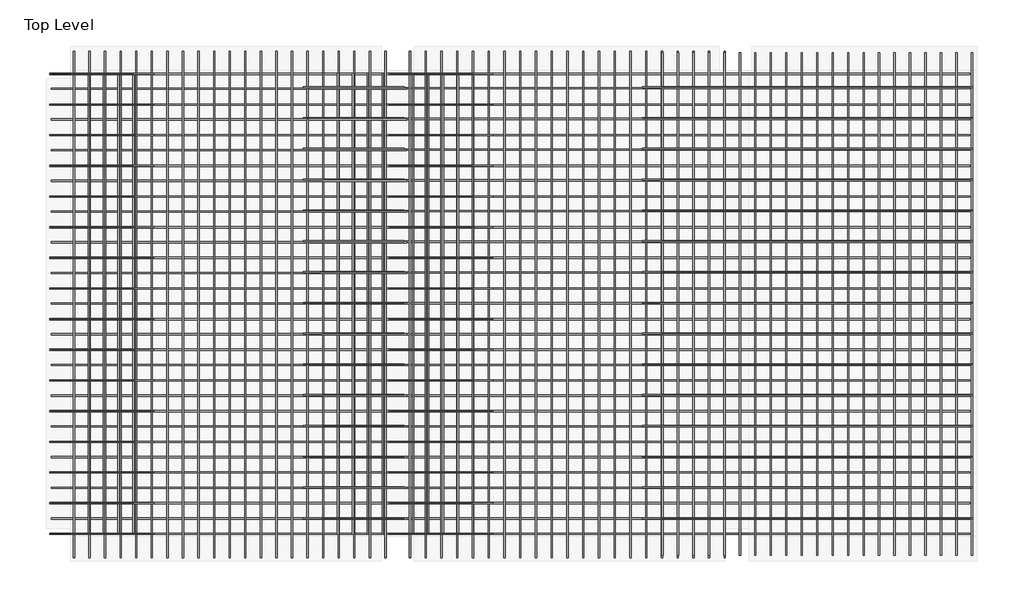
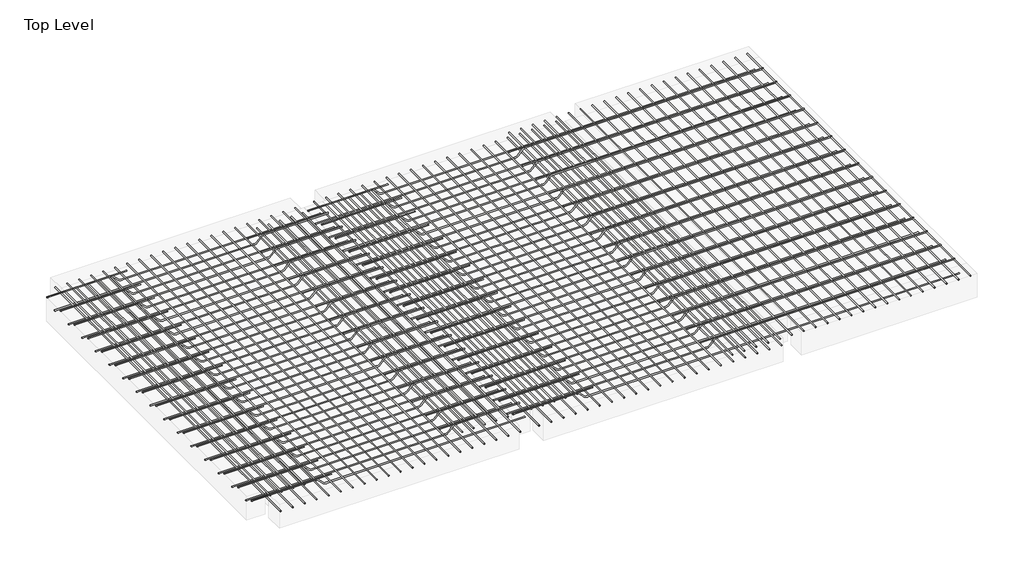
# One storey, part 2 of 2: 14 reinforcing bars.
"""IFC4 building model written with IfcOpenShell, lengths in millimetres."""

from ifc_helpers import new_model, si_unit, point, frame, origin, place, context, project, spatial, polyline, circle_curve, trimmed, segment, composite_curve, source, transform, mapped, element, save
from ifc_brep_helpers import swept_disk

model = new_model("IFC4")

# Units and contexts
model_context = context("Model", 3, world=origin())
ifc_project = project(units=[si_unit("LENGTHUNIT", "METRE", prefix="MILLI")], contexts=[model_context])

# Site, building, storey
site = spatial("IfcSite", under=ifc_project)
building = spatial("IfcBuilding", under=site)
storey = spatial("IfcBuildingStorey", under=building, Name="Top Level", Elevation=12801.6)

# Reinforcing bars
placement = place(None, origin())
reinforcing_bar_shape = source(origin(), model_context, "Body", "SolidModel", [
    swept_disk(composite_curve([segment(polyline([(-9347.5125695, 4803.6334631, 12770.6), (-8565.5792829, 4803.6334631, 12770.6)]), True, "CONTINUOUS"), segment(trimmed(circle_curve(frame((-8565.5792829, 4803.6334631, 12724.6), z_axis=(0.0, 1.0, 0.0), x_axis=(0.0, 0.0, 46.0)), 46.0), [point((-8565.5792829, 4803.6334631, 12770.6))], [point((-8533.052371, 4803.6334631, 12757.1269119))], True, "CARTESIAN"), True, "CONTINUOUS"), segment(polyline([(-8533.052371, 4803.6334631, 12757.1269119), (-8469.5985471, 4803.6334631, 12693.6730881)]), True, "CONTINUOUS"), segment(trimmed(circle_curve(frame((-8437.0716352, 4803.6334631, 12726.2), z_axis=(0.0, -1.0000000000000002, 0.0), x_axis=(-32.526911900000414, 0.0, -32.526911900000414)), 46.0), [point((-8469.5985471, 4803.6334631, 12693.6730881))], [point((-8437.0716352, 4803.6334631, 12680.2))], True, "CARTESIAN"), True, "CONTINUOUS"), segment(polyline([(-8437.0716352, 4803.6334631, 12680.2), (-5982.0597449, 4803.6334631, 12680.2)]), True, "CONTINUOUS")], self_intersect=False), 6.0),
])
element("IfcReinforcingBar", 1, at=placement, inside=storey, context=model_context, shape_type="MappedRepresentation", body=[
    mapped(reinforcing_bar_shape, transform((0.0, 0.0, 0.0), x_axis=(1.0, 0.0, 0.0), y_axis=(0.0, 1.0, 0.0), z_axis=(0.0, 0.0, 1.0))),
    mapped(reinforcing_bar_shape, transform((0.0, -290.5066667, 0.0), x_axis=(1.0, 0.0, 0.0), y_axis=(0.0, 1.0, 0.0), z_axis=(0.0, 0.0, 1.0))),
    mapped(reinforcing_bar_shape, transform((0.0, -581.0133333, 0.0), x_axis=(1.0, 0.0, 0.0), y_axis=(0.0, 1.0, 0.0), z_axis=(0.0, 0.0, 1.0))),
    mapped(reinforcing_bar_shape, transform((0.0, -871.52, 0.0), x_axis=(1.0, 0.0, 0.0), y_axis=(0.0, 1.0, 0.0), z_axis=(0.0, 0.0, 1.0))),
    mapped(reinforcing_bar_shape, transform((0.0, -1162.0266667, 0.0), x_axis=(1.0, 0.0, 0.0), y_axis=(0.0, 1.0, 0.0), z_axis=(0.0, 0.0, 1.0))),
    mapped(reinforcing_bar_shape, transform((0.0, -1452.5333333, 0.0), x_axis=(1.0, 0.0, 0.0), y_axis=(0.0, 1.0, 0.0), z_axis=(0.0, 0.0, 1.0))),
    mapped(reinforcing_bar_shape, transform((0.0, -1743.04, 0.0), x_axis=(1.0, 0.0, 0.0), y_axis=(0.0, 1.0, 0.0), z_axis=(0.0, 0.0, 1.0))),
    mapped(reinforcing_bar_shape, transform((0.0, -2033.5466667, 0.0), x_axis=(1.0, 0.0, 0.0), y_axis=(0.0, 1.0, 0.0), z_axis=(0.0, 0.0, 1.0))),
    mapped(reinforcing_bar_shape, transform((0.0, -2324.0533333, 0.0), x_axis=(1.0, 0.0, 0.0), y_axis=(0.0, 1.0, 0.0), z_axis=(0.0, 0.0, 1.0))),
    mapped(reinforcing_bar_shape, transform((0.0, -2614.56, 0.0), x_axis=(1.0, 0.0, 0.0), y_axis=(0.0, 1.0, 0.0), z_axis=(0.0, 0.0, 1.0))),
    mapped(reinforcing_bar_shape, transform((0.0, -2905.0666667, 0.0), x_axis=(1.0, 0.0, 0.0), y_axis=(0.0, 1.0, 0.0), z_axis=(0.0, 0.0, 1.0))),
    mapped(reinforcing_bar_shape, transform((0.0, -3195.5733333, 0.0), x_axis=(1.0, 0.0, 0.0), y_axis=(0.0, 1.0, 0.0), z_axis=(0.0, 0.0, 1.0))),
    mapped(reinforcing_bar_shape, transform((0.0, -3486.08, 0.0), x_axis=(1.0, 0.0, 0.0), y_axis=(0.0, 1.0, 0.0), z_axis=(0.0, 0.0, 1.0))),
    mapped(reinforcing_bar_shape, transform((0.0, -3776.5866667, 0.0), x_axis=(1.0, 0.0, 0.0), y_axis=(0.0, 1.0, 0.0), z_axis=(0.0, 0.0, 1.0))),
    mapped(reinforcing_bar_shape, transform((0.0, -4067.0933333, 0.0), x_axis=(1.0, 0.0, 0.0), y_axis=(0.0, 1.0, 0.0), z_axis=(0.0, 0.0, 1.0))),
    mapped(reinforcing_bar_shape, transform((0.0, -4357.6, 0.0), x_axis=(1.0, 0.0, 0.0), y_axis=(0.0, 1.0, 0.0), z_axis=(0.0, 0.0, 1.0))),
])
reinforcing_bar_2_shape = source(origin(), model_context, "Body", "SolidModel", [
    swept_disk(composite_curve([segment(polyline([(-5968.6109354, 590.4513536, 12770.6), (-6750.544222, 590.4513536, 12770.6)]), True, "CONTINUOUS"), segment(trimmed(circle_curve(frame((-6750.544222, 590.4513536, 12724.6), z_axis=(0.0, -1.0, 0.0), x_axis=(0.0, 0.0, 46.0)), 46.0), [point((-6750.544222, 590.4513536, 12770.6))], [point((-6783.0711339, 590.4513536, 12757.1269119))], True, "CARTESIAN"), True, "CONTINUOUS"), segment(polyline([(-6783.0711339, 590.4513536, 12757.1269119), (-6846.5249578, 590.4513536, 12693.6730881)]), True, "CONTINUOUS"), segment(trimmed(circle_curve(frame((-6879.0518697, 590.4513536, 12726.2), z_axis=(0.0, 1.0000000000000002, 0.0), x_axis=(32.526911899999504, 0.0, -32.526911900000414)), 46.0), [point((-6846.5249578, 590.4513536, 12693.6730881))], [point((-6879.0518697, 590.4513536, 12680.2))], True, "CARTESIAN"), True, "CONTINUOUS"), segment(polyline([(-6879.0518697, 590.4513536, 12680.2), (-9334.06376, 590.4513536, 12680.2)]), True, "CONTINUOUS")], self_intersect=False), 6.0),
])
element("IfcReinforcingBar", 2, at=placement, inside=storey, context=model_context, shape_type="MappedRepresentation", body=[
    mapped(reinforcing_bar_2_shape, transform((0.0, 0.0, 0.0), x_axis=(1.0, 0.0, 0.0), y_axis=(0.0, 1.0, 0.0), z_axis=(0.0, 0.0, 1.0))),
    mapped(reinforcing_bar_2_shape, transform((0.0, 290.9296088, 0.0), x_axis=(1.0, 0.0, 0.0), y_axis=(0.0, 1.0, 0.0), z_axis=(0.0, 0.0, 1.0))),
    mapped(reinforcing_bar_2_shape, transform((0.0, 581.8592177, 0.0), x_axis=(1.0, 0.0, 0.0), y_axis=(0.0, 1.0, 0.0), z_axis=(0.0, 0.0, 1.0))),
    mapped(reinforcing_bar_2_shape, transform((0.0, 872.7888265, 0.0), x_axis=(1.0, 0.0, 0.0), y_axis=(0.0, 1.0, 0.0), z_axis=(0.0, 0.0, 1.0))),
    mapped(reinforcing_bar_2_shape, transform((0.0, 1163.7184353, 0.0), x_axis=(1.0, 0.0, 0.0), y_axis=(0.0, 1.0, 0.0), z_axis=(0.0, 0.0, 1.0))),
    mapped(reinforcing_bar_2_shape, transform((0.0, 1454.6480442, 0.0), x_axis=(1.0, 0.0, 0.0), y_axis=(0.0, 1.0, 0.0), z_axis=(0.0, 0.0, 1.0))),
    mapped(reinforcing_bar_2_shape, transform((0.0, 1745.577653, 0.0), x_axis=(1.0, 0.0, 0.0), y_axis=(0.0, 1.0, 0.0), z_axis=(0.0, 0.0, 1.0))),
    mapped(reinforcing_bar_2_shape, transform((0.0, 2036.5072618, 0.0), x_axis=(1.0, 0.0, 0.0), y_axis=(0.0, 1.0, 0.0), z_axis=(0.0, 0.0, 1.0))),
    mapped(reinforcing_bar_2_shape, transform((0.0, 2327.4368707, 0.0), x_axis=(1.0, 0.0, 0.0), y_axis=(0.0, 1.0, 0.0), z_axis=(0.0, 0.0, 1.0))),
    mapped(reinforcing_bar_2_shape, transform((0.0, 2618.3664795, 0.0), x_axis=(1.0, 0.0, 0.0), y_axis=(0.0, 1.0, 0.0), z_axis=(0.0, 0.0, 1.0))),
    mapped(reinforcing_bar_2_shape, transform((0.0, 2909.2960883, 0.0), x_axis=(1.0, 0.0, 0.0), y_axis=(0.0, 1.0, 0.0), z_axis=(0.0, 0.0, 1.0))),
    mapped(reinforcing_bar_2_shape, transform((0.0, 3200.2256972, 0.0), x_axis=(1.0, 0.0, 0.0), y_axis=(0.0, 1.0, 0.0), z_axis=(0.0, 0.0, 1.0))),
    mapped(reinforcing_bar_2_shape, transform((0.0, 3491.155306, 0.0), x_axis=(1.0, 0.0, 0.0), y_axis=(0.0, 1.0, 0.0), z_axis=(0.0, 0.0, 1.0))),
    mapped(reinforcing_bar_2_shape, transform((0.0, 3782.0849148, 0.0), x_axis=(1.0, 0.0, 0.0), y_axis=(0.0, 1.0, 0.0), z_axis=(0.0, 0.0, 1.0))),
    mapped(reinforcing_bar_2_shape, transform((0.0, 4073.0145236, 0.0), x_axis=(1.0, 0.0, 0.0), y_axis=(0.0, 1.0, 0.0), z_axis=(0.0, 0.0, 1.0))),
])
reinforcing_bar_3_shape = source(origin(), model_context, "Body", "SolidModel", [
    swept_disk(composite_curve([segment(polyline([(-8556.5984173, 4809.6334631, 12760.3006995), (-8556.5984173, 440.0334631, 12760.3006995)]), True, "CONTINUOUS")], self_intersect=False), 6.0),
])
element("IfcReinforcingBar", 3, at=placement, inside=storey, context=model_context, shape_type="MappedRepresentation", body=[
    mapped(reinforcing_bar_3_shape, transform((0.0, 0.0, 0.0), x_axis=(1.0, 0.0, 0.0), y_axis=(0.0, 1.0, 0.0), z_axis=(0.0, 0.0, 1.0))),
    mapped(reinforcing_bar_3_shape, transform((-140.6783338, 0.0, 0.0), x_axis=(1.0, 0.0, 0.0), y_axis=(0.0, 1.0, 0.0), z_axis=(0.0, 0.0, 1.0))),
    mapped(reinforcing_bar_3_shape, transform((-281.3566676, 0.0, 0.0), x_axis=(1.0, 0.0, 0.0), y_axis=(0.0, 1.0, 0.0), z_axis=(0.0, 0.0, 1.0))),
    mapped(reinforcing_bar_3_shape, transform((-422.0350014, 0.0, 0.0), x_axis=(1.0, 0.0, 0.0), y_axis=(0.0, 1.0, 0.0), z_axis=(0.0, 0.0, 1.0))),
    mapped(reinforcing_bar_3_shape, transform((-562.7133352, 0.0, 0.0), x_axis=(1.0, 0.0, 0.0), y_axis=(0.0, 1.0, 0.0), z_axis=(0.0, 0.0, 1.0))),
])
reinforcing_bar_4_shape = source(origin(), model_context, "Body", "SolidModel", [
    swept_disk(composite_curve([segment(polyline([(-6759.5250876, 4809.6334631, 12760.3006995), (-6759.5250876, 440.0334631, 12760.3006995)]), True, "CONTINUOUS")], self_intersect=False), 6.0),
])
element("IfcReinforcingBar", 4, at=placement, inside=storey, context=model_context, shape_type="MappedRepresentation", body=[
    mapped(reinforcing_bar_4_shape, transform((0.0, 0.0, 0.0), x_axis=(1.0, 0.0, 0.0), y_axis=(0.0, 1.0, 0.0), z_axis=(0.0, 0.0, 1.0))),
    mapped(reinforcing_bar_4_shape, transform((140.6783338, 0.0, 0.0), x_axis=(1.0, 0.0, 0.0), y_axis=(0.0, 1.0, 0.0), z_axis=(0.0, 0.0, 1.0))),
    mapped(reinforcing_bar_4_shape, transform((281.3566676, 0.0, 0.0), x_axis=(1.0, 0.0, 0.0), y_axis=(0.0, 1.0, 0.0), z_axis=(0.0, 0.0, 1.0))),
    mapped(reinforcing_bar_4_shape, transform((422.0350014, 0.0, 0.0), x_axis=(1.0, 0.0, 0.0), y_axis=(0.0, 1.0, 0.0), z_axis=(0.0, 0.0, 1.0))),
    mapped(reinforcing_bar_4_shape, transform((562.7133352, 0.0, 0.0), x_axis=(1.0, 0.0, 0.0), y_axis=(0.0, 1.0, 0.0), z_axis=(0.0, 0.0, 1.0))),
])
reinforcing_bar_5_shape = source(origin(), model_context, "Body", "SolidModel", [
    swept_disk(composite_curve([segment(polyline([(-9338.4522926, 4805.6334631, 12772.6), (-8365.7369752, 4805.6334631, 12772.6)]), True, "CONTINUOUS")], self_intersect=False), 4.0),
])
element("IfcReinforcingBar", 5, at=placement, inside=storey, context=model_context, shape_type="MappedRepresentation", body=[
    mapped(reinforcing_bar_5_shape, transform((0.0, 0.0, 0.0), x_axis=(1.0, 0.0, 0.0), y_axis=(0.0, 1.0, 0.0), z_axis=(0.0, 0.0, 1.0))),
    mapped(reinforcing_bar_5_shape, transform((0.0, -290.7733333, 0.0), x_axis=(1.0, 0.0, 0.0), y_axis=(0.0, 1.0, 0.0), z_axis=(0.0, 0.0, 1.0))),
    mapped(reinforcing_bar_5_shape, transform((0.0, -581.5466667, 0.0), x_axis=(1.0, 0.0, 0.0), y_axis=(0.0, 1.0, 0.0), z_axis=(0.0, 0.0, 1.0))),
    mapped(reinforcing_bar_5_shape, transform((0.0, -872.32, 0.0), x_axis=(1.0, 0.0, 0.0), y_axis=(0.0, 1.0, 0.0), z_axis=(0.0, 0.0, 1.0))),
    mapped(reinforcing_bar_5_shape, transform((0.0, -1163.0933333, 0.0), x_axis=(1.0, 0.0, 0.0), y_axis=(0.0, 1.0, 0.0), z_axis=(0.0, 0.0, 1.0))),
    mapped(reinforcing_bar_5_shape, transform((0.0, -1453.8666667, 0.0), x_axis=(1.0, 0.0, 0.0), y_axis=(0.0, 1.0, 0.0), z_axis=(0.0, 0.0, 1.0))),
    mapped(reinforcing_bar_5_shape, transform((0.0, -1744.64, 0.0), x_axis=(1.0, 0.0, 0.0), y_axis=(0.0, 1.0, 0.0), z_axis=(0.0, 0.0, 1.0))),
    mapped(reinforcing_bar_5_shape, transform((0.0, -2035.4133333, 0.0), x_axis=(1.0, 0.0, 0.0), y_axis=(0.0, 1.0, 0.0), z_axis=(0.0, 0.0, 1.0))),
    mapped(reinforcing_bar_5_shape, transform((0.0, -2326.1866667, 0.0), x_axis=(1.0, 0.0, 0.0), y_axis=(0.0, 1.0, 0.0), z_axis=(0.0, 0.0, 1.0))),
    mapped(reinforcing_bar_5_shape, transform((0.0, -2616.96, 0.0), x_axis=(1.0, 0.0, 0.0), y_axis=(0.0, 1.0, 0.0), z_axis=(0.0, 0.0, 1.0))),
    mapped(reinforcing_bar_5_shape, transform((0.0, -2907.7333333, 0.0), x_axis=(1.0, 0.0, 0.0), y_axis=(0.0, 1.0, 0.0), z_axis=(0.0, 0.0, 1.0))),
    mapped(reinforcing_bar_5_shape, transform((0.0, -3198.5066667, 0.0), x_axis=(1.0, 0.0, 0.0), y_axis=(0.0, 1.0, 0.0), z_axis=(0.0, 0.0, 1.0))),
    mapped(reinforcing_bar_5_shape, transform((0.0, -3489.28, 0.0), x_axis=(1.0, 0.0, 0.0), y_axis=(0.0, 1.0, 0.0), z_axis=(0.0, 0.0, 1.0))),
    mapped(reinforcing_bar_5_shape, transform((0.0, -3780.0533333, 0.0), x_axis=(1.0, 0.0, 0.0), y_axis=(0.0, 1.0, 0.0), z_axis=(0.0, 0.0, 1.0))),
    mapped(reinforcing_bar_5_shape, transform((0.0, -4070.8266667, 0.0), x_axis=(1.0, 0.0, 0.0), y_axis=(0.0, 1.0, 0.0), z_axis=(0.0, 0.0, 1.0))),
    mapped(reinforcing_bar_5_shape, transform((0.0, -4361.6, 0.0), x_axis=(1.0, 0.0, 0.0), y_axis=(0.0, 1.0, 0.0), z_axis=(0.0, 0.0, 1.0))),
])
reinforcing_bar_6_shape = source(origin(), model_context, "Body", "SolidModel", [
    swept_disk(composite_curve([segment(polyline([(-5991.3123639, 4678.4115375, 12772.6), (-6950.3865297, 4678.4115375, 12772.6)]), True, "CONTINUOUS")], self_intersect=False), 4.0),
])
element("IfcReinforcingBar", 6, at=placement, inside=storey, context=model_context, shape_type="MappedRepresentation", body=[
    mapped(reinforcing_bar_6_shape, transform((0.0, 0.0, 0.0), x_axis=(1.0, 0.0, 0.0), y_axis=(0.0, 1.0, 0.0), z_axis=(0.0, 0.0, 1.0))),
    mapped(reinforcing_bar_6_shape, transform((0.0, -291.8025106, 0.0), x_axis=(1.0, 0.0, 0.0), y_axis=(0.0, 1.0, 0.0), z_axis=(0.0, 0.0, 1.0))),
    mapped(reinforcing_bar_6_shape, transform((0.0, -583.6050212, 0.0), x_axis=(1.0, 0.0, 0.0), y_axis=(0.0, 1.0, 0.0), z_axis=(0.0, 0.0, 1.0))),
    mapped(reinforcing_bar_6_shape, transform((0.0, -875.4075319, 0.0), x_axis=(1.0, 0.0, 0.0), y_axis=(0.0, 1.0, 0.0), z_axis=(0.0, 0.0, 1.0))),
    mapped(reinforcing_bar_6_shape, transform((0.0, -1167.2100425, 0.0), x_axis=(1.0, 0.0, 0.0), y_axis=(0.0, 1.0, 0.0), z_axis=(0.0, 0.0, 1.0))),
    mapped(reinforcing_bar_6_shape, transform((0.0, -1459.0125531, 0.0), x_axis=(1.0, 0.0, 0.0), y_axis=(0.0, 1.0, 0.0), z_axis=(0.0, 0.0, 1.0))),
    mapped(reinforcing_bar_6_shape, transform((0.0, -1750.8150637, 0.0), x_axis=(1.0, 0.0, 0.0), y_axis=(0.0, 1.0, 0.0), z_axis=(0.0, 0.0, 1.0))),
    mapped(reinforcing_bar_6_shape, transform((0.0, -2042.6175743, 0.0), x_axis=(1.0, 0.0, 0.0), y_axis=(0.0, 1.0, 0.0), z_axis=(0.0, 0.0, 1.0))),
    mapped(reinforcing_bar_6_shape, transform((0.0, -2334.420085, 0.0), x_axis=(1.0, 0.0, 0.0), y_axis=(0.0, 1.0, 0.0), z_axis=(0.0, 0.0, 1.0))),
    mapped(reinforcing_bar_6_shape, transform((0.0, -2626.2225956, 0.0), x_axis=(1.0, 0.0, 0.0), y_axis=(0.0, 1.0, 0.0), z_axis=(0.0, 0.0, 1.0))),
    mapped(reinforcing_bar_6_shape, transform((0.0, -2918.0251062, 0.0), x_axis=(1.0, 0.0, 0.0), y_axis=(0.0, 1.0, 0.0), z_axis=(0.0, 0.0, 1.0))),
    mapped(reinforcing_bar_6_shape, transform((0.0, -3209.8276168, 0.0), x_axis=(1.0, 0.0, 0.0), y_axis=(0.0, 1.0, 0.0), z_axis=(0.0, 0.0, 1.0))),
    mapped(reinforcing_bar_6_shape, transform((0.0, -3501.6301274, 0.0), x_axis=(1.0, 0.0, 0.0), y_axis=(0.0, 1.0, 0.0), z_axis=(0.0, 0.0, 1.0))),
    mapped(reinforcing_bar_6_shape, transform((0.0, -3793.4326381, 0.0), x_axis=(1.0, 0.0, 0.0), y_axis=(0.0, 1.0, 0.0), z_axis=(0.0, 0.0, 1.0))),
    mapped(reinforcing_bar_6_shape, transform((0.0, -4085.2351487, 0.0), x_axis=(1.0, 0.0, 0.0), y_axis=(0.0, 1.0, 0.0), z_axis=(0.0, 0.0, 1.0))),
])
reinforcing_bar_7_shape = source(origin(), model_context, "Body", "SolidModel", [
    swept_disk(composite_curve([segment(polyline([(-6169.8117524, 218.9117605, 12688.7387401), (-6169.8117524, 5019.9992064, 12688.7387401)]), True, "CONTINUOUS")], self_intersect=False), 6.0),
])
element("IfcReinforcingBar", 7, at=placement, inside=storey, context=model_context, shape_type="MappedRepresentation", body=[
    mapped(reinforcing_bar_7_shape, transform((0.0, 0.0, 0.0), x_axis=(1.0, 0.0, 0.0), y_axis=(0.0, 1.0, 0.0), z_axis=(0.0, 0.0, 1.0))),
    mapped(reinforcing_bar_7_shape, transform((-147.475, 0.0, 0.0), x_axis=(1.0, 0.0, 0.0), y_axis=(0.0, 1.0, 0.0), z_axis=(0.0, 0.0, 1.0))),
    mapped(reinforcing_bar_7_shape, transform((-294.95, 0.0, 0.0), x_axis=(1.0, 0.0, 0.0), y_axis=(0.0, 1.0, 0.0), z_axis=(0.0, 0.0, 1.0))),
    mapped(reinforcing_bar_7_shape, transform((-442.425, 0.0, 0.0), x_axis=(1.0, 0.0, 0.0), y_axis=(0.0, 1.0, 0.0), z_axis=(0.0, 0.0, 1.0))),
    mapped(reinforcing_bar_7_shape, transform((-589.9, 0.0, 0.0), x_axis=(1.0, 0.0, 0.0), y_axis=(0.0, 1.0, 0.0), z_axis=(0.0, 0.0, 1.0))),
    mapped(reinforcing_bar_7_shape, transform((-737.375, 0.0, 0.0), x_axis=(1.0, 0.0, 0.0), y_axis=(0.0, 1.0, 0.0), z_axis=(0.0, 0.0, 1.0))),
    mapped(reinforcing_bar_7_shape, transform((-884.85, 0.0, 0.0), x_axis=(1.0, 0.0, 0.0), y_axis=(0.0, 1.0, 0.0), z_axis=(0.0, 0.0, 1.0))),
    mapped(reinforcing_bar_7_shape, transform((-1032.325, 0.0, 0.0), x_axis=(1.0, 0.0, 0.0), y_axis=(0.0, 1.0, 0.0), z_axis=(0.0, 0.0, 1.0))),
    mapped(reinforcing_bar_7_shape, transform((-1179.8, 0.0, 0.0), x_axis=(1.0, 0.0, 0.0), y_axis=(0.0, 1.0, 0.0), z_axis=(0.0, 0.0, 1.0))),
    mapped(reinforcing_bar_7_shape, transform((-1327.275, 0.0, 0.0), x_axis=(1.0, 0.0, 0.0), y_axis=(0.0, 1.0, 0.0), z_axis=(0.0, 0.0, 1.0))),
    mapped(reinforcing_bar_7_shape, transform((-1474.75, 0.0, 0.0), x_axis=(1.0, 0.0, 0.0), y_axis=(0.0, 1.0, 0.0), z_axis=(0.0, 0.0, 1.0))),
    mapped(reinforcing_bar_7_shape, transform((-1622.225, 0.0, 0.0), x_axis=(1.0, 0.0, 0.0), y_axis=(0.0, 1.0, 0.0), z_axis=(0.0, 0.0, 1.0))),
    mapped(reinforcing_bar_7_shape, transform((-1769.7, 0.0, 0.0), x_axis=(1.0, 0.0, 0.0), y_axis=(0.0, 1.0, 0.0), z_axis=(0.0, 0.0, 1.0))),
    mapped(reinforcing_bar_7_shape, transform((-1917.175, 0.0, 0.0), x_axis=(1.0, 0.0, 0.0), y_axis=(0.0, 1.0, 0.0), z_axis=(0.0, 0.0, 1.0))),
    mapped(reinforcing_bar_7_shape, transform((-2064.65, 0.0, 0.0), x_axis=(1.0, 0.0, 0.0), y_axis=(0.0, 1.0, 0.0), z_axis=(0.0, 0.0, 1.0))),
    mapped(reinforcing_bar_7_shape, transform((-2212.125, 0.0, 0.0), x_axis=(1.0, 0.0, 0.0), y_axis=(0.0, 1.0, 0.0), z_axis=(0.0, 0.0, 1.0))),
    mapped(reinforcing_bar_7_shape, transform((-2359.6, 0.0, 0.0), x_axis=(1.0, 0.0, 0.0), y_axis=(0.0, 1.0, 0.0), z_axis=(0.0, 0.0, 1.0))),
    mapped(reinforcing_bar_7_shape, transform((-2507.075, 0.0, 0.0), x_axis=(1.0, 0.0, 0.0), y_axis=(0.0, 1.0, 0.0), z_axis=(0.0, 0.0, 1.0))),
    mapped(reinforcing_bar_7_shape, transform((-2654.55, 0.0, 0.0), x_axis=(1.0, 0.0, 0.0), y_axis=(0.0, 1.0, 0.0), z_axis=(0.0, 0.0, 1.0))),
    mapped(reinforcing_bar_7_shape, transform((-2802.025, 0.0, 0.0), x_axis=(1.0, 0.0, 0.0), y_axis=(0.0, 1.0, 0.0), z_axis=(0.0, 0.0, 1.0))),
    mapped(reinforcing_bar_7_shape, transform((-2949.5, 0.0, 0.0), x_axis=(1.0, 0.0, 0.0), y_axis=(0.0, 1.0, 0.0), z_axis=(0.0, 0.0, 1.0))),
])
reinforcing_bar_8_shape = source(origin(), model_context, "Body", "SolidModel", [
    swept_disk(composite_curve([segment(polyline([(-6134.4125695, 4803.6334631, 12770.6), (-5352.4792829, 4803.6334631, 12770.6)]), True, "CONTINUOUS"), segment(trimmed(circle_curve(frame((-5352.4792829, 4803.6334631, 12724.6), z_axis=(0.0, 1.0, 0.0), x_axis=(0.0, 0.0, 46.0)), 46.0), [point((-5352.4792829, 4803.6334631, 12770.6))], [point((-5319.952371, 4803.6334631, 12757.1269119))], True, "CARTESIAN"), True, "CONTINUOUS"), segment(polyline([(-5319.952371, 4803.6334631, 12757.1269119), (-5256.4985471, 4803.6334631, 12693.6730881)]), True, "CONTINUOUS"), segment(trimmed(circle_curve(frame((-5223.9716352, 4803.6334631, 12726.2), z_axis=(0.0, -1.0, 0.0), x_axis=(-32.526911900000414, 0.0, -32.526911900000414)), 46.0), [point((-5256.4985471, 4803.6334631, 12693.6730881))], [point((-5223.9716352, 4803.6334631, 12680.2))], True, "CARTESIAN"), True, "CONTINUOUS"), segment(polyline([(-5223.9716352, 4803.6334631, 12680.2), (-639.5382507, 4803.6334631, 12680.2)]), True, "CONTINUOUS")], self_intersect=False), 6.0),
])
element("IfcReinforcingBar", 8, at=placement, inside=storey, context=model_context, shape_type="MappedRepresentation", body=[
    mapped(reinforcing_bar_8_shape, transform((0.0, 0.0, 0.0), x_axis=(1.0, 0.0, 0.0), y_axis=(0.0, 1.0, 0.0), z_axis=(0.0, 0.0, 1.0))),
    mapped(reinforcing_bar_8_shape, transform((0.0, -290.5066667, 0.0), x_axis=(1.0, 0.0, 0.0), y_axis=(0.0, 1.0, 0.0), z_axis=(0.0, 0.0, 1.0))),
    mapped(reinforcing_bar_8_shape, transform((0.0, -581.0133333, 0.0), x_axis=(1.0, 0.0, 0.0), y_axis=(0.0, 1.0, 0.0), z_axis=(0.0, 0.0, 1.0))),
    mapped(reinforcing_bar_8_shape, transform((0.0, -871.52, 0.0), x_axis=(1.0, 0.0, 0.0), y_axis=(0.0, 1.0, 0.0), z_axis=(0.0, 0.0, 1.0))),
    mapped(reinforcing_bar_8_shape, transform((0.0, -1162.0266667, 0.0), x_axis=(1.0, 0.0, 0.0), y_axis=(0.0, 1.0, 0.0), z_axis=(0.0, 0.0, 1.0))),
    mapped(reinforcing_bar_8_shape, transform((0.0, -1452.5333333, 0.0), x_axis=(1.0, 0.0, 0.0), y_axis=(0.0, 1.0, 0.0), z_axis=(0.0, 0.0, 1.0))),
    mapped(reinforcing_bar_8_shape, transform((0.0, -1743.04, 0.0), x_axis=(1.0, 0.0, 0.0), y_axis=(0.0, 1.0, 0.0), z_axis=(0.0, 0.0, 1.0))),
    mapped(reinforcing_bar_8_shape, transform((0.0, -2033.5466667, 0.0), x_axis=(1.0, 0.0, 0.0), y_axis=(0.0, 1.0, 0.0), z_axis=(0.0, 0.0, 1.0))),
    mapped(reinforcing_bar_8_shape, transform((0.0, -2324.0533333, 0.0), x_axis=(1.0, 0.0, 0.0), y_axis=(0.0, 1.0, 0.0), z_axis=(0.0, 0.0, 1.0))),
    mapped(reinforcing_bar_8_shape, transform((0.0, -2614.56, 0.0), x_axis=(1.0, 0.0, 0.0), y_axis=(0.0, 1.0, 0.0), z_axis=(0.0, 0.0, 1.0))),
    mapped(reinforcing_bar_8_shape, transform((0.0, -2905.0666667, 0.0), x_axis=(1.0, 0.0, 0.0), y_axis=(0.0, 1.0, 0.0), z_axis=(0.0, 0.0, 1.0))),
    mapped(reinforcing_bar_8_shape, transform((0.0, -3195.5733333, 0.0), x_axis=(1.0, 0.0, 0.0), y_axis=(0.0, 1.0, 0.0), z_axis=(0.0, 0.0, 1.0))),
    mapped(reinforcing_bar_8_shape, transform((0.0, -3486.08, 0.0), x_axis=(1.0, 0.0, 0.0), y_axis=(0.0, 1.0, 0.0), z_axis=(0.0, 0.0, 1.0))),
    mapped(reinforcing_bar_8_shape, transform((0.0, -3776.5866667, 0.0), x_axis=(1.0, 0.0, 0.0), y_axis=(0.0, 1.0, 0.0), z_axis=(0.0, 0.0, 1.0))),
    mapped(reinforcing_bar_8_shape, transform((0.0, -4067.0933333, 0.0), x_axis=(1.0, 0.0, 0.0), y_axis=(0.0, 1.0, 0.0), z_axis=(0.0, 0.0, 1.0))),
    mapped(reinforcing_bar_8_shape, transform((0.0, -4357.6, 0.0), x_axis=(1.0, 0.0, 0.0), y_axis=(0.0, 1.0, 0.0), z_axis=(0.0, 0.0, 1.0))),
])
reinforcing_bar_9_shape = source(origin(), model_context, "Body", "SolidModel", [
    swept_disk(composite_curve([segment(polyline([(-634.9311577, 590.4513536, 12770.6), (-3537.444222, 590.4513536, 12770.6)]), True, "CONTINUOUS"), segment(trimmed(circle_curve(frame((-3537.444222, 590.4513536, 12724.6), z_axis=(0.0, -1.0, 0.0), x_axis=(0.0, 0.0, 46.0)), 46.0), [point((-3537.444222, 590.4513536, 12770.6))], [point((-3569.9711339, 590.4513536, 12757.1269119))], True, "CARTESIAN"), True, "CONTINUOUS"), segment(polyline([(-3569.9711339, 590.4513536, 12757.1269119), (-3633.4249578, 590.4513536, 12693.6730881)]), True, "CONTINUOUS"), segment(trimmed(circle_curve(frame((-3665.9518697, 590.4513536, 12726.2), z_axis=(0.0, 1.0, 0.0), x_axis=(32.52691189999996, 0.0, -32.526911900000414)), 46.0), [point((-3633.4249578, 590.4513536, 12693.6730881))], [point((-3665.9518697, 590.4513536, 12680.2))], True, "CARTESIAN"), True, "CONTINUOUS"), segment(polyline([(-3665.9518697, 590.4513536, 12680.2), (-6120.96376, 590.4513536, 12680.2)]), True, "CONTINUOUS")], self_intersect=False), 6.0),
])
element("IfcReinforcingBar", 9, at=placement, inside=storey, context=model_context, shape_type="MappedRepresentation", body=[
    mapped(reinforcing_bar_9_shape, transform((0.0, 0.0, 0.0), x_axis=(1.0, 0.0, 0.0), y_axis=(0.0, 1.0, 0.0), z_axis=(0.0, 0.0, 1.0))),
    mapped(reinforcing_bar_9_shape, transform((0.0, 291.2629007, 0.0), x_axis=(1.0, 0.0, 0.0), y_axis=(0.0, 1.0, 0.0), z_axis=(0.0, 0.0, 1.0))),
    mapped(reinforcing_bar_9_shape, transform((0.0, 582.5258014, 0.0), x_axis=(1.0, 0.0, 0.0), y_axis=(0.0, 1.0, 0.0), z_axis=(0.0, 0.0, 1.0))),
    mapped(reinforcing_bar_9_shape, transform((0.0, 873.7887021, 0.0), x_axis=(1.0, 0.0, 0.0), y_axis=(0.0, 1.0, 0.0), z_axis=(0.0, 0.0, 1.0))),
    mapped(reinforcing_bar_9_shape, transform((0.0, 1165.0516028, 0.0), x_axis=(1.0, 0.0, 0.0), y_axis=(0.0, 1.0, 0.0), z_axis=(0.0, 0.0, 1.0))),
    mapped(reinforcing_bar_9_shape, transform((0.0, 1456.3145035, 0.0), x_axis=(1.0, 0.0, 0.0), y_axis=(0.0, 1.0, 0.0), z_axis=(0.0, 0.0, 1.0))),
    mapped(reinforcing_bar_9_shape, transform((0.0, 1747.5774042, 0.0), x_axis=(1.0, 0.0, 0.0), y_axis=(0.0, 1.0, 0.0), z_axis=(0.0, 0.0, 1.0))),
    mapped(reinforcing_bar_9_shape, transform((0.0, 2038.8403049, 0.0), x_axis=(1.0, 0.0, 0.0), y_axis=(0.0, 1.0, 0.0), z_axis=(0.0, 0.0, 1.0))),
    mapped(reinforcing_bar_9_shape, transform((0.0, 2330.1032056, 0.0), x_axis=(1.0, 0.0, 0.0), y_axis=(0.0, 1.0, 0.0), z_axis=(0.0, 0.0, 1.0))),
    mapped(reinforcing_bar_9_shape, transform((0.0, 2621.3661063, 0.0), x_axis=(1.0, 0.0, 0.0), y_axis=(0.0, 1.0, 0.0), z_axis=(0.0, 0.0, 1.0))),
    mapped(reinforcing_bar_9_shape, transform((0.0, 2912.629007, 0.0), x_axis=(1.0, 0.0, 0.0), y_axis=(0.0, 1.0, 0.0), z_axis=(0.0, 0.0, 1.0))),
    mapped(reinforcing_bar_9_shape, transform((0.0, 3203.8919077, 0.0), x_axis=(1.0, 0.0, 0.0), y_axis=(0.0, 1.0, 0.0), z_axis=(0.0, 0.0, 1.0))),
    mapped(reinforcing_bar_9_shape, transform((0.0, 3495.1548084, 0.0), x_axis=(1.0, 0.0, 0.0), y_axis=(0.0, 1.0, 0.0), z_axis=(0.0, 0.0, 1.0))),
    mapped(reinforcing_bar_9_shape, transform((0.0, 3786.4177091, 0.0), x_axis=(1.0, 0.0, 0.0), y_axis=(0.0, 1.0, 0.0), z_axis=(0.0, 0.0, 1.0))),
    mapped(reinforcing_bar_9_shape, transform((0.0, 4077.6806098, 0.0), x_axis=(1.0, 0.0, 0.0), y_axis=(0.0, 1.0, 0.0), z_axis=(0.0, 0.0, 1.0))),
])
reinforcing_bar_10_shape = source(origin(), model_context, "Body", "SolidModel", [
    swept_disk(composite_curve([segment(polyline([(-3546.4250876, 5003.4291982, 12760.3006995), (-3546.4250876, 243.4585871, 12760.3006995)]), True, "CONTINUOUS")], self_intersect=False), 6.0),
])
element("IfcReinforcingBar", 10, at=placement, inside=storey, context=model_context, shape_type="MappedRepresentation", body=[
    mapped(reinforcing_bar_10_shape, transform((0.0, 0.0, 0.0), x_axis=(1.0, 0.0, 0.0), y_axis=(0.0, 1.0, 0.0), z_axis=(0.0, 0.0, 1.0))),
    mapped(reinforcing_bar_10_shape, transform((146.4369665, 0.0, 0.0), x_axis=(1.0, 0.0, 0.0), y_axis=(0.0, 1.0, 0.0), z_axis=(0.0, 0.0, 1.0))),
    mapped(reinforcing_bar_10_shape, transform((292.8739331, 0.0, 0.0), x_axis=(1.0, 0.0, 0.0), y_axis=(0.0, 1.0, 0.0), z_axis=(0.0, 0.0, 1.0))),
    mapped(reinforcing_bar_10_shape, transform((439.3108996, 0.0, 0.0), x_axis=(1.0, 0.0, 0.0), y_axis=(0.0, 1.0, 0.0), z_axis=(0.0, 0.0, 1.0))),
    mapped(reinforcing_bar_10_shape, transform((585.7478661, 0.0, 0.0), x_axis=(1.0, 0.0, 0.0), y_axis=(0.0, 1.0, 0.0), z_axis=(0.0, 0.0, 1.0))),
    mapped(reinforcing_bar_10_shape, transform((732.1848326, 0.0, 0.0), x_axis=(1.0, 0.0, 0.0), y_axis=(0.0, 1.0, 0.0), z_axis=(0.0, 0.0, 1.0))),
    mapped(reinforcing_bar_10_shape, transform((878.6217992, 0.0, 0.0), x_axis=(1.0, 0.0, 0.0), y_axis=(0.0, 1.0, 0.0), z_axis=(0.0, 0.0, 1.0))),
    mapped(reinforcing_bar_10_shape, transform((1025.0587657, 0.0, 0.0), x_axis=(1.0, 0.0, 0.0), y_axis=(0.0, 1.0, 0.0), z_axis=(0.0, 0.0, 1.0))),
    mapped(reinforcing_bar_10_shape, transform((1171.4957322, 0.0, 0.0), x_axis=(1.0, 0.0, 0.0), y_axis=(0.0, 1.0, 0.0), z_axis=(0.0, 0.0, 1.0))),
    mapped(reinforcing_bar_10_shape, transform((1317.9326988, 0.0, 0.0), x_axis=(1.0, 0.0, 0.0), y_axis=(0.0, 1.0, 0.0), z_axis=(0.0, 0.0, 1.0))),
    mapped(reinforcing_bar_10_shape, transform((1464.3696653, 0.0, 0.0), x_axis=(1.0, 0.0, 0.0), y_axis=(0.0, 1.0, 0.0), z_axis=(0.0, 0.0, 1.0))),
    mapped(reinforcing_bar_10_shape, transform((1610.8066318, 0.0, 0.0), x_axis=(1.0, 0.0, 0.0), y_axis=(0.0, 1.0, 0.0), z_axis=(0.0, 0.0, 1.0))),
    mapped(reinforcing_bar_10_shape, transform((1757.2435983, 0.0, 0.0), x_axis=(1.0, 0.0, 0.0), y_axis=(0.0, 1.0, 0.0), z_axis=(0.0, 0.0, 1.0))),
    mapped(reinforcing_bar_10_shape, transform((1903.6805649, 0.0, 0.0), x_axis=(1.0, 0.0, 0.0), y_axis=(0.0, 1.0, 0.0), z_axis=(0.0, 0.0, 1.0))),
    mapped(reinforcing_bar_10_shape, transform((2050.1175314, 0.0, 0.0), x_axis=(1.0, 0.0, 0.0), y_axis=(0.0, 1.0, 0.0), z_axis=(0.0, 0.0, 1.0))),
    mapped(reinforcing_bar_10_shape, transform((2196.5544979, 0.0, 0.0), x_axis=(1.0, 0.0, 0.0), y_axis=(0.0, 1.0, 0.0), z_axis=(0.0, 0.0, 1.0))),
    mapped(reinforcing_bar_10_shape, transform((2342.9914645, 0.0, 0.0), x_axis=(1.0, 0.0, 0.0), y_axis=(0.0, 1.0, 0.0), z_axis=(0.0, 0.0, 1.0))),
    mapped(reinforcing_bar_10_shape, transform((2489.428431, 0.0, 0.0), x_axis=(1.0, 0.0, 0.0), y_axis=(0.0, 1.0, 0.0), z_axis=(0.0, 0.0, 1.0))),
    mapped(reinforcing_bar_10_shape, transform((2635.8653975, 0.0, 0.0), x_axis=(1.0, 0.0, 0.0), y_axis=(0.0, 1.0, 0.0), z_axis=(0.0, 0.0, 1.0))),
    mapped(reinforcing_bar_10_shape, transform((2782.302364, 0.0, 0.0), x_axis=(1.0, 0.0, 0.0), y_axis=(0.0, 1.0, 0.0), z_axis=(0.0, 0.0, 1.0))),
    mapped(reinforcing_bar_10_shape, transform((2928.7393306, 0.0, 0.0), x_axis=(1.0, 0.0, 0.0), y_axis=(0.0, 1.0, 0.0), z_axis=(0.0, 0.0, 1.0))),
])
reinforcing_bar_11_shape = source(origin(), model_context, "Body", "SolidModel", [
    swept_disk(composite_curve([segment(polyline([(-6125.3522926, 4805.6334631, 12772.6), (-5152.6369752, 4805.6334631, 12772.6)]), True, "CONTINUOUS")], self_intersect=False), 4.0),
])
element("IfcReinforcingBar", 11, at=placement, inside=storey, context=model_context, shape_type="MappedRepresentation", body=[
    mapped(reinforcing_bar_11_shape, transform((0.0, 0.0, 0.0), x_axis=(1.0, 0.0, 0.0), y_axis=(0.0, 1.0, 0.0), z_axis=(0.0, 0.0, 1.0))),
    mapped(reinforcing_bar_11_shape, transform((0.0, -290.7733333, 0.0), x_axis=(1.0, 0.0, 0.0), y_axis=(0.0, 1.0, 0.0), z_axis=(0.0, 0.0, 1.0))),
    mapped(reinforcing_bar_11_shape, transform((0.0, -581.5466667, 0.0), x_axis=(1.0, 0.0, 0.0), y_axis=(0.0, 1.0, 0.0), z_axis=(0.0, 0.0, 1.0))),
    mapped(reinforcing_bar_11_shape, transform((0.0, -872.32, 0.0), x_axis=(1.0, 0.0, 0.0), y_axis=(0.0, 1.0, 0.0), z_axis=(0.0, 0.0, 1.0))),
    mapped(reinforcing_bar_11_shape, transform((0.0, -1163.0933333, 0.0), x_axis=(1.0, 0.0, 0.0), y_axis=(0.0, 1.0, 0.0), z_axis=(0.0, 0.0, 1.0))),
    mapped(reinforcing_bar_11_shape, transform((0.0, -1453.8666667, 0.0), x_axis=(1.0, 0.0, 0.0), y_axis=(0.0, 1.0, 0.0), z_axis=(0.0, 0.0, 1.0))),
    mapped(reinforcing_bar_11_shape, transform((0.0, -1744.64, 0.0), x_axis=(1.0, 0.0, 0.0), y_axis=(0.0, 1.0, 0.0), z_axis=(0.0, 0.0, 1.0))),
    mapped(reinforcing_bar_11_shape, transform((0.0, -2035.4133333, 0.0), x_axis=(1.0, 0.0, 0.0), y_axis=(0.0, 1.0, 0.0), z_axis=(0.0, 0.0, 1.0))),
    mapped(reinforcing_bar_11_shape, transform((0.0, -2326.1866667, 0.0), x_axis=(1.0, 0.0, 0.0), y_axis=(0.0, 1.0, 0.0), z_axis=(0.0, 0.0, 1.0))),
    mapped(reinforcing_bar_11_shape, transform((0.0, -2616.96, 0.0), x_axis=(1.0, 0.0, 0.0), y_axis=(0.0, 1.0, 0.0), z_axis=(0.0, 0.0, 1.0))),
    mapped(reinforcing_bar_11_shape, transform((0.0, -2907.7333333, 0.0), x_axis=(1.0, 0.0, 0.0), y_axis=(0.0, 1.0, 0.0), z_axis=(0.0, 0.0, 1.0))),
    mapped(reinforcing_bar_11_shape, transform((0.0, -3198.5066667, 0.0), x_axis=(1.0, 0.0, 0.0), y_axis=(0.0, 1.0, 0.0), z_axis=(0.0, 0.0, 1.0))),
    mapped(reinforcing_bar_11_shape, transform((0.0, -3489.28, 0.0), x_axis=(1.0, 0.0, 0.0), y_axis=(0.0, 1.0, 0.0), z_axis=(0.0, 0.0, 1.0))),
    mapped(reinforcing_bar_11_shape, transform((0.0, -3780.0533333, 0.0), x_axis=(1.0, 0.0, 0.0), y_axis=(0.0, 1.0, 0.0), z_axis=(0.0, 0.0, 1.0))),
    mapped(reinforcing_bar_11_shape, transform((0.0, -4070.8266667, 0.0), x_axis=(1.0, 0.0, 0.0), y_axis=(0.0, 1.0, 0.0), z_axis=(0.0, 0.0, 1.0))),
    mapped(reinforcing_bar_11_shape, transform((0.0, -4361.6, 0.0), x_axis=(1.0, 0.0, 0.0), y_axis=(0.0, 1.0, 0.0), z_axis=(0.0, 0.0, 1.0))),
])
reinforcing_bar_12_shape = source(origin(), model_context, "Body", "SolidModel", [
    swept_disk(composite_curve([segment(polyline([(-610.8785317, 4678.4115375, 12772.6), (-3737.2865297, 4678.4115375, 12772.6)]), True, "CONTINUOUS")], self_intersect=False), 4.0),
])
element("IfcReinforcingBar", 12, at=placement, inside=storey, context=model_context, shape_type="MappedRepresentation", body=[
    mapped(reinforcing_bar_12_shape, transform((0.0, 0.0, 0.0), x_axis=(1.0, 0.0, 0.0), y_axis=(0.0, 1.0, 0.0), z_axis=(0.0, 0.0, 1.0))),
    mapped(reinforcing_bar_12_shape, transform((0.0, -291.8025106, 0.0), x_axis=(1.0, 0.0, 0.0), y_axis=(0.0, 1.0, 0.0), z_axis=(0.0, 0.0, 1.0))),
    mapped(reinforcing_bar_12_shape, transform((0.0, -583.6050212, 0.0), x_axis=(1.0, 0.0, 0.0), y_axis=(0.0, 1.0, 0.0), z_axis=(0.0, 0.0, 1.0))),
    mapped(reinforcing_bar_12_shape, transform((0.0, -875.4075319, 0.0), x_axis=(1.0, 0.0, 0.0), y_axis=(0.0, 1.0, 0.0), z_axis=(0.0, 0.0, 1.0))),
    mapped(reinforcing_bar_12_shape, transform((0.0, -1167.2100425, 0.0), x_axis=(1.0, 0.0, 0.0), y_axis=(0.0, 1.0, 0.0), z_axis=(0.0, 0.0, 1.0))),
    mapped(reinforcing_bar_12_shape, transform((0.0, -1459.0125531, 0.0), x_axis=(1.0, 0.0, 0.0), y_axis=(0.0, 1.0, 0.0), z_axis=(0.0, 0.0, 1.0))),
    mapped(reinforcing_bar_12_shape, transform((0.0, -1750.8150637, 0.0), x_axis=(1.0, 0.0, 0.0), y_axis=(0.0, 1.0, 0.0), z_axis=(0.0, 0.0, 1.0))),
    mapped(reinforcing_bar_12_shape, transform((0.0, -2042.6175743, 0.0), x_axis=(1.0, 0.0, 0.0), y_axis=(0.0, 1.0, 0.0), z_axis=(0.0, 0.0, 1.0))),
    mapped(reinforcing_bar_12_shape, transform((0.0, -2334.420085, 0.0), x_axis=(1.0, 0.0, 0.0), y_axis=(0.0, 1.0, 0.0), z_axis=(0.0, 0.0, 1.0))),
    mapped(reinforcing_bar_12_shape, transform((0.0, -2626.2225956, 0.0), x_axis=(1.0, 0.0, 0.0), y_axis=(0.0, 1.0, 0.0), z_axis=(0.0, 0.0, 1.0))),
    mapped(reinforcing_bar_12_shape, transform((0.0, -2918.0251062, 0.0), x_axis=(1.0, 0.0, 0.0), y_axis=(0.0, 1.0, 0.0), z_axis=(0.0, 0.0, 1.0))),
    mapped(reinforcing_bar_12_shape, transform((0.0, -3209.8276168, 0.0), x_axis=(1.0, 0.0, 0.0), y_axis=(0.0, 1.0, 0.0), z_axis=(0.0, 0.0, 1.0))),
    mapped(reinforcing_bar_12_shape, transform((0.0, -3501.6301274, 0.0), x_axis=(1.0, 0.0, 0.0), y_axis=(0.0, 1.0, 0.0), z_axis=(0.0, 0.0, 1.0))),
    mapped(reinforcing_bar_12_shape, transform((0.0, -3793.4326381, 0.0), x_axis=(1.0, 0.0, 0.0), y_axis=(0.0, 1.0, 0.0), z_axis=(0.0, 0.0, 1.0))),
    mapped(reinforcing_bar_12_shape, transform((0.0, -4085.2351487, 0.0), x_axis=(1.0, 0.0, 0.0), y_axis=(0.0, 1.0, 0.0), z_axis=(0.0, 0.0, 1.0))),
])
reinforcing_bar_13_shape = source(origin(), model_context, "Body", "SolidModel", [
    swept_disk(composite_curve([segment(polyline([(-2956.7117524, 218.9117605, 12688.7387401), (-2956.7117524, 5019.9992064, 12688.7387401)]), True, "CONTINUOUS")], self_intersect=False), 6.0),
])
element("IfcReinforcingBar", 13, at=placement, inside=storey, context=model_context, shape_type="MappedRepresentation", body=[
    mapped(reinforcing_bar_13_shape, transform((0.0, 0.0, 0.0), x_axis=(1.0, 0.0, 0.0), y_axis=(0.0, 1.0, 0.0), z_axis=(0.0, 0.0, 1.0))),
    mapped(reinforcing_bar_13_shape, transform((-149.025, 0.0, 0.0), x_axis=(1.0, 0.0, 0.0), y_axis=(0.0, 1.0, 0.0), z_axis=(0.0, 0.0, 1.0))),
    mapped(reinforcing_bar_13_shape, transform((-298.05, 0.0, 0.0), x_axis=(1.0, 0.0, 0.0), y_axis=(0.0, 1.0, 0.0), z_axis=(0.0, 0.0, 1.0))),
    mapped(reinforcing_bar_13_shape, transform((-447.075, 0.0, 0.0), x_axis=(1.0, 0.0, 0.0), y_axis=(0.0, 1.0, 0.0), z_axis=(0.0, 0.0, 1.0))),
    mapped(reinforcing_bar_13_shape, transform((-596.1, 0.0, 0.0), x_axis=(1.0, 0.0, 0.0), y_axis=(0.0, 1.0, 0.0), z_axis=(0.0, 0.0, 1.0))),
    mapped(reinforcing_bar_13_shape, transform((-745.125, 0.0, 0.0), x_axis=(1.0, 0.0, 0.0), y_axis=(0.0, 1.0, 0.0), z_axis=(0.0, 0.0, 1.0))),
    mapped(reinforcing_bar_13_shape, transform((-894.15, 0.0, 0.0), x_axis=(1.0, 0.0, 0.0), y_axis=(0.0, 1.0, 0.0), z_axis=(0.0, 0.0, 1.0))),
    mapped(reinforcing_bar_13_shape, transform((-1043.175, 0.0, 0.0), x_axis=(1.0, 0.0, 0.0), y_axis=(0.0, 1.0, 0.0), z_axis=(0.0, 0.0, 1.0))),
    mapped(reinforcing_bar_13_shape, transform((-1192.2, 0.0, 0.0), x_axis=(1.0, 0.0, 0.0), y_axis=(0.0, 1.0, 0.0), z_axis=(0.0, 0.0, 1.0))),
    mapped(reinforcing_bar_13_shape, transform((-1341.225, 0.0, 0.0), x_axis=(1.0, 0.0, 0.0), y_axis=(0.0, 1.0, 0.0), z_axis=(0.0, 0.0, 1.0))),
    mapped(reinforcing_bar_13_shape, transform((-1490.25, 0.0, 0.0), x_axis=(1.0, 0.0, 0.0), y_axis=(0.0, 1.0, 0.0), z_axis=(0.0, 0.0, 1.0))),
    mapped(reinforcing_bar_13_shape, transform((-1639.275, 0.0, 0.0), x_axis=(1.0, 0.0, 0.0), y_axis=(0.0, 1.0, 0.0), z_axis=(0.0, 0.0, 1.0))),
    mapped(reinforcing_bar_13_shape, transform((-1788.3, 0.0, 0.0), x_axis=(1.0, 0.0, 0.0), y_axis=(0.0, 1.0, 0.0), z_axis=(0.0, 0.0, 1.0))),
    mapped(reinforcing_bar_13_shape, transform((-1937.325, 0.0, 0.0), x_axis=(1.0, 0.0, 0.0), y_axis=(0.0, 1.0, 0.0), z_axis=(0.0, 0.0, 1.0))),
    mapped(reinforcing_bar_13_shape, transform((-2086.35, 0.0, 0.0), x_axis=(1.0, 0.0, 0.0), y_axis=(0.0, 1.0, 0.0), z_axis=(0.0, 0.0, 1.0))),
    mapped(reinforcing_bar_13_shape, transform((-2235.375, 0.0, 0.0), x_axis=(1.0, 0.0, 0.0), y_axis=(0.0, 1.0, 0.0), z_axis=(0.0, 0.0, 1.0))),
    mapped(reinforcing_bar_13_shape, transform((-2384.4, 0.0, 0.0), x_axis=(1.0, 0.0, 0.0), y_axis=(0.0, 1.0, 0.0), z_axis=(0.0, 0.0, 1.0))),
    mapped(reinforcing_bar_13_shape, transform((-2533.425, 0.0, 0.0), x_axis=(1.0, 0.0, 0.0), y_axis=(0.0, 1.0, 0.0), z_axis=(0.0, 0.0, 1.0))),
    mapped(reinforcing_bar_13_shape, transform((-2682.45, 0.0, 0.0), x_axis=(1.0, 0.0, 0.0), y_axis=(0.0, 1.0, 0.0), z_axis=(0.0, 0.0, 1.0))),
    mapped(reinforcing_bar_13_shape, transform((-2831.475, 0.0, 0.0), x_axis=(1.0, 0.0, 0.0), y_axis=(0.0, 1.0, 0.0), z_axis=(0.0, 0.0, 1.0))),
    mapped(reinforcing_bar_13_shape, transform((-2980.5, 0.0, 0.0), x_axis=(1.0, 0.0, 0.0), y_axis=(0.0, 1.0, 0.0), z_axis=(0.0, 0.0, 1.0))),
])
reinforcing_bar_14_shape = source(origin(), model_context, "Body", "SolidModel", [
    swept_disk(composite_curve([segment(polyline([(-5343.4984173, 4809.6334631, 12760.3006995), (-5343.4984173, 440.0334631, 12760.3006995)]), True, "CONTINUOUS")], self_intersect=False), 6.0),
])
element("IfcReinforcingBar", 14, at=placement, inside=storey, context=model_context, shape_type="MappedRepresentation", body=[
    mapped(reinforcing_bar_14_shape, transform((0.0, 0.0, 0.0), x_axis=(1.0, 0.0, 0.0), y_axis=(0.0, 1.0, 0.0), z_axis=(0.0, 0.0, 1.0))),
    mapped(reinforcing_bar_14_shape, transform((-140.6783338, 0.0, 0.0), x_axis=(1.0, 0.0, 0.0), y_axis=(0.0, 1.0, 0.0), z_axis=(0.0, 0.0, 1.0))),
    mapped(reinforcing_bar_14_shape, transform((-281.3566676, 0.0, 0.0), x_axis=(1.0, 0.0, 0.0), y_axis=(0.0, 1.0, 0.0), z_axis=(0.0, 0.0, 1.0))),
    mapped(reinforcing_bar_14_shape, transform((-422.0350014, 0.0, 0.0), x_axis=(1.0, 0.0, 0.0), y_axis=(0.0, 1.0, 0.0), z_axis=(0.0, 0.0, 1.0))),
    mapped(reinforcing_bar_14_shape, transform((-562.7133352, 0.0, 0.0), x_axis=(1.0, 0.0, 0.0), y_axis=(0.0, 1.0, 0.0), z_axis=(0.0, 0.0, 1.0))),
])

save(model, "model.ifc")

# Revit data of these elements
# Elements 1, 2, 3, 4, 5, 6, 7, 8, 9, 10, 11, 12, 13, 14 (IfcReinforcingBar)
#   Phase Created = New Construction
